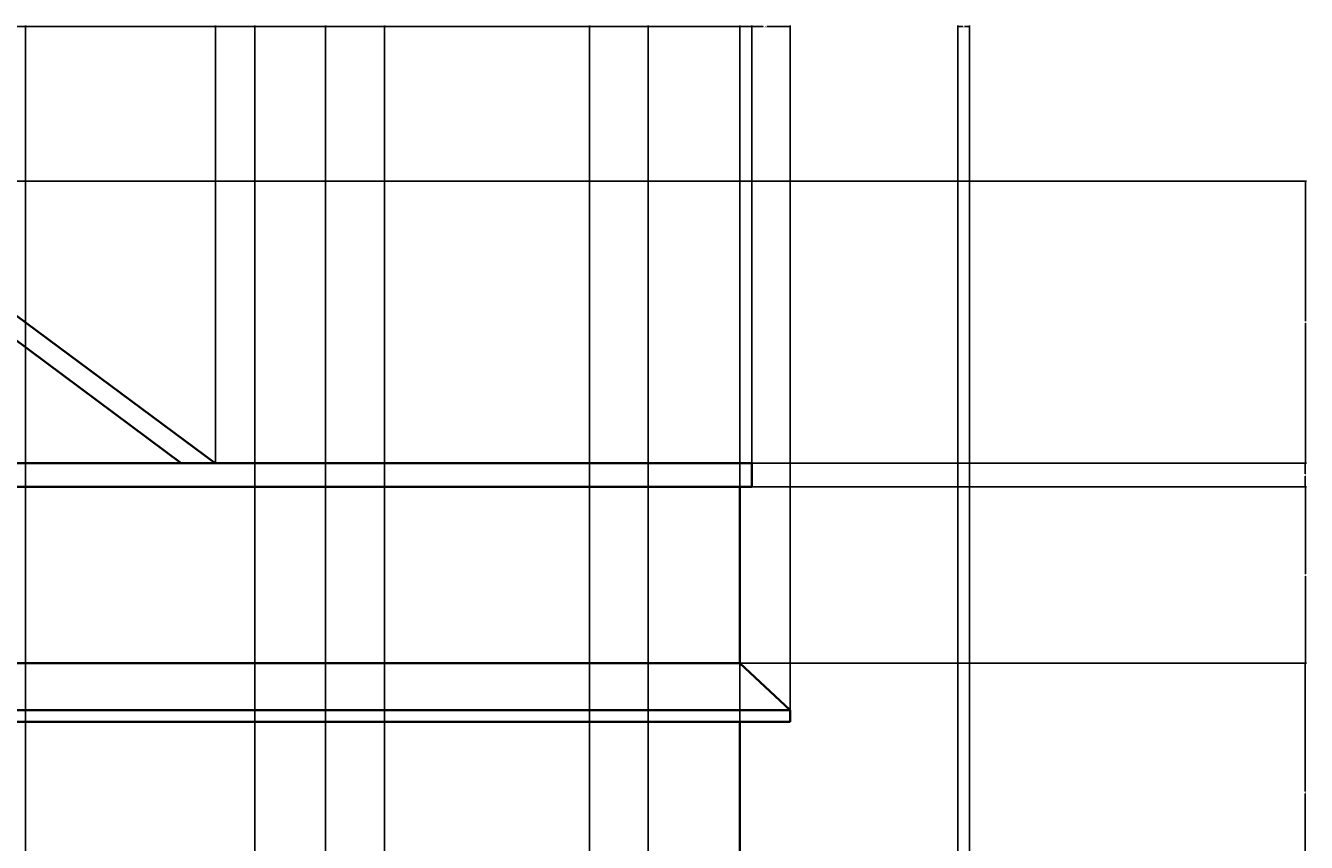
# Model space of a CAD drawing. Units: inches. Extents: x 1817 to 2378, y 1915 to 2370.
# Tile 8 of 8: x 2160 to 2377, y 2231 to 2370. Entities that reach past the tile are written whole.
import ezdxf

# ---------------------------------------------------------------- set-up
doc = ezdxf.new("R2010")
doc.units = ezdxf.units.IN
doc.layers.add('A-ANNO-DIMS', color=2, linetype='Continuous', lineweight=18)
doc.layers.add('A-ELEV', color=7, linetype='Continuous', lineweight=35)
doc.styles.get("Standard").update_dxf_attribs({"font": 'arial.ttf'})
doc.dimstyles.get("Standard").update_dxf_attribs({"dimtxt": 0.18, "dimasz": 0.18, "dimexe": 0.18, "dimexo": 0.0625, "dimgap": 0.09, "dimtad": 0, "dimtih": 1, "dimtoh": 1, "dimdec": 4, "dimzin": 0, "dimdsep": 46, "dimtxsty": 'Standard', "dimcen": 0.09, "dimadec": 0, "dimazin": 0, "dimtfac": 1, "dimtdec": 4, "dimtofl": 0, "dimtmove": 0, "dimatfit": 3, "dimfxl": 1, "dimtolj": 1, "dimtzin": 0, "dimarcsym": 0})

# ---------------------------------------------------------------- blocks, each defined once
blk = doc.blocks.new('*D36')
at = {"layer": 'A-ANNO-DIMS', "color": 0, "lineweight": -2, "transparency": 16777216}
for p, q in [((2159.62, 2217.96), (2159.62, 2369.94)), ((2159.8, 2369.76), (2178.71, 2369.76)), ((2198.41, 2369.76), (2179.5, 2369.76)), ((2198.59, 2156.58), (2198.59, 2369.94))]:
    blk.add_line(p, q, dxfattribs=at)
at = {"layer": 'A-ANNO-DIMS', "color": 0, "transparency": 16777216}
for points in [[(2159.8, 2369.79), (2159.8, 2369.73), (2159.62, 2369.76)], [(2198.41, 2369.79), (2198.41, 2369.73), (2198.59, 2369.76)]]:
    blk.add_solid(points, dxfattribs=at)
at = {"layer": 'Defpoints', "color": 0, "transparency": 16777216}
for p in [(2198.59, 2369.76), (2159.62, 2217.9), (2198.59, 2156.51)]:
    blk.add_point(p, dxfattribs=at)
at = {"layer": 'A-ANNO-DIMS', "color": 0, "transparency": 16777216, "insert": (2179.1, 2369.76), "char_height": 0.18, "attachment_point": 5}
blk.add_mtext('\\A1;38.97', dxfattribs=at)
blk = doc.blocks.new('*D37')
at = {"layer": 'A-ANNO-DIMS', "color": 0, "lineweight": -2, "transparency": 16777216}
for p, q in [((2198.59, 2156.58), (2198.59, 2369.94)), ((2198.77, 2369.76), (2204.15, 2369.76)), ((2210.44, 2369.76), (2205.06, 2369.76)), ((2210.62, 2217.57), (2210.62, 2369.94))]:
    blk.add_line(p, q, dxfattribs=at)
at = {"layer": 'A-ANNO-DIMS', "color": 0, "transparency": 16777216}
for points in [[(2198.77, 2369.79), (2198.77, 2369.73), (2198.59, 2369.76)], [(2210.44, 2369.79), (2210.44, 2369.73), (2210.62, 2369.76)]]:
    blk.add_solid(points, dxfattribs=at)
at = {"layer": 'Defpoints', "color": 0, "transparency": 16777216}
for p in [(2210.62, 2369.76), (2210.62, 2217.51), (2198.59, 2156.51)]:
    blk.add_point(p, dxfattribs=at)
at = {"layer": 'A-ANNO-DIMS', "color": 0, "transparency": 16777216, "insert": (2204.6, 2369.76), "char_height": 0.18, "attachment_point": 5}
blk.add_mtext('\\A1;12.027', dxfattribs=at)
blk = doc.blocks.new('*D38')
at = {"layer": 'A-ANNO-DIMS', "color": 0, "lineweight": -2, "transparency": 16777216}
for p, q in [((2210.62, 2217.57), (2210.62, 2369.94)), ((2210.8, 2369.76), (2215.41, 2369.76)), ((2220.44, 2369.76), (2215.83, 2369.76)), ((2220.62, 2136.11), (2220.62, 2369.94))]:
    blk.add_line(p, q, dxfattribs=at)
at = {"layer": 'A-ANNO-DIMS', "color": 0, "transparency": 16777216}
for points in [[(2210.8, 2369.79), (2210.8, 2369.73), (2210.62, 2369.76)], [(2220.44, 2369.79), (2220.44, 2369.73), (2220.62, 2369.76)]]:
    blk.add_solid(points, dxfattribs=at)
at = {"layer": 'Defpoints', "color": 0, "transparency": 16777216}
for p in [(2220.62, 2369.76), (2210.62, 2217.51), (2220.62, 2136.04)]:
    blk.add_point(p, dxfattribs=at)
at = {"layer": 'A-ANNO-DIMS', "color": 0, "transparency": 16777216, "insert": (2215.62, 2369.76), "char_height": 0.18, "attachment_point": 5}
blk.add_mtext('\\A1;10', dxfattribs=at)
blk = doc.blocks.new('*D39')
at = {"layer": 'A-ANNO-DIMS', "color": 0, "lineweight": -2, "transparency": 16777216}
for p, q in [((2220.62, 2136.11), (2220.62, 2369.94)), ((2220.8, 2369.76), (2237.66, 2369.76)), ((2255.31, 2369.76), (2238.45, 2369.76)), ((2255.49, 2136.11), (2255.49, 2369.94))]:
    blk.add_line(p, q, dxfattribs=at)
at = {"layer": 'A-ANNO-DIMS', "color": 0, "transparency": 16777216}
for points in [[(2220.8, 2369.79), (2220.8, 2369.73), (2220.62, 2369.76)], [(2255.31, 2369.79), (2255.31, 2369.73), (2255.49, 2369.76)]]:
    blk.add_solid(points, dxfattribs=at)
at = {"layer": 'Defpoints', "color": 0, "transparency": 16777216}
for p in [(2255.49, 2369.76), (2220.62, 2136.04), (2255.49, 2136.04)]:
    blk.add_point(p, dxfattribs=at)
at = {"layer": 'A-ANNO-DIMS', "color": 0, "transparency": 16777216, "insert": (2238.05, 2369.76), "char_height": 0.18, "attachment_point": 5}
blk.add_mtext('\\A1;34.87', dxfattribs=at)
blk = doc.blocks.new('*D40')
at = {"layer": 'A-ANNO-DIMS', "color": 0, "lineweight": -2, "transparency": 16777216}
for p, q in [((2255.49, 2136.11), (2255.49, 2369.94)), ((2255.67, 2369.76), (2260.28, 2369.76)), ((2265.31, 2369.76), (2260.7, 2369.76)), ((2265.49, 2217.57), (2265.49, 2369.94))]:
    blk.add_line(p, q, dxfattribs=at)
at = {"layer": 'A-ANNO-DIMS', "color": 0, "transparency": 16777216}
for points in [[(2255.67, 2369.79), (2255.67, 2369.73), (2255.49, 2369.76)], [(2265.31, 2369.79), (2265.31, 2369.73), (2265.49, 2369.76)]]:
    blk.add_solid(points, dxfattribs=at)
at = {"layer": 'Defpoints', "color": 0, "transparency": 16777216}
for p in [(2265.49, 2369.76), (2265.49, 2217.51), (2255.49, 2136.04)]:
    blk.add_point(p, dxfattribs=at)
at = {"layer": 'A-ANNO-DIMS', "color": 0, "transparency": 16777216, "insert": (2260.49, 2369.76), "char_height": 0.18, "attachment_point": 5}
blk.add_mtext('\\A1;10', dxfattribs=at)
blk = doc.blocks.new('*D41')
at = {"layer": 'A-ANNO-DIMS', "color": 0, "lineweight": -2, "transparency": 16777216}
for p, q in [((2318.11, 2103.63), (2318.11, 2369.94)), ((2318.29, 2369.76), (2318.96, 2369.76)), ((2319.93, 2369.76), (2319.26, 2369.76)), ((2320.11, 2156.58), (2320.11, 2369.94))]:
    blk.add_line(p, q, dxfattribs=at)
at = {"layer": 'A-ANNO-DIMS', "color": 0, "transparency": 16777216}
for points in [[(2318.29, 2369.79), (2318.29, 2369.73), (2318.11, 2369.76)], [(2319.93, 2369.79), (2319.93, 2369.73), (2320.11, 2369.76)]]:
    blk.add_solid(points, dxfattribs=at)
at = {"layer": 'Defpoints', "color": 0, "transparency": 16777216}
for p in [(2320.11, 2369.76), (2320.11, 2156.51), (2318.11, 2103.57)]:
    blk.add_point(p, dxfattribs=at)
at = {"layer": 'A-ANNO-DIMS', "color": 0, "transparency": 16777216, "insert": (2319.11, 2369.76), "char_height": 0.18, "attachment_point": 5}
blk.add_mtext('\\A1;2', dxfattribs=at)
blk = doc.blocks.new('*D47')
at = {"layer": 'A-ANNO-DIMS', "color": 0, "lineweight": -2, "transparency": 16777216}
for p, q in [((2127.08, 2343.57), (2127.08, 2369.94)), ((2127.26, 2369.76), (2159.09, 2369.76)), ((2191.7, 2369.76), (2159.87, 2369.76)), ((2191.88, 2295.57), (2191.88, 2369.94))]:
    blk.add_line(p, q, dxfattribs=at)
at = {"layer": 'A-ANNO-DIMS', "color": 0, "transparency": 16777216}
for points in [[(2127.26, 2369.79), (2127.26, 2369.73), (2127.08, 2369.76)], [(2191.7, 2369.79), (2191.7, 2369.73), (2191.88, 2369.76)]]:
    blk.add_solid(points, dxfattribs=at)
at = {"layer": 'Defpoints', "color": 0, "transparency": 16777216}
for p in [(2191.88, 2369.76), (2127.08, 2343.51), (2191.88, 2295.51)]:
    blk.add_point(p, dxfattribs=at)
at = {"layer": 'A-ANNO-DIMS', "color": 0, "transparency": 16777216, "insert": (2159.48, 2369.76), "char_height": 0.18, "attachment_point": 5}
blk.add_mtext('\\A1;64.79', dxfattribs=at)
blk = doc.blocks.new('*D48')
at = {"layer": 'A-ANNO-DIMS', "color": 0, "lineweight": -2, "transparency": 16777216}
for p, q in [((2191.88, 2295.57), (2191.88, 2369.94)), ((2192.06, 2369.76), (2236.1, 2369.76)), ((2280.9, 2369.76), (2236.86, 2369.76)), ((2281.08, 2291.57), (2281.08, 2369.94))]:
    blk.add_line(p, q, dxfattribs=at)
at = {"layer": 'A-ANNO-DIMS', "color": 0, "transparency": 16777216}
for points in [[(2192.06, 2369.79), (2192.06, 2369.73), (2191.88, 2369.76)], [(2280.9, 2369.79), (2280.9, 2369.73), (2281.08, 2369.76)]]:
    blk.add_solid(points, dxfattribs=at)
at = {"layer": 'Defpoints', "color": 0, "transparency": 16777216}
for p in [(2281.08, 2369.76), (2191.88, 2295.51), (2281.08, 2291.51)]:
    blk.add_point(p, dxfattribs=at)
at = {"layer": 'A-ANNO-DIMS', "color": 0, "transparency": 16777216, "insert": (2236.48, 2369.76), "char_height": 0.18, "attachment_point": 5}
blk.add_mtext('\\A1;89.21', dxfattribs=at)
blk = doc.blocks.new('*D49')
at = {"layer": 'A-ANNO-DIMS', "color": 0, "lineweight": -2, "transparency": 16777216}
for p, q in [((2281.08, 2291.57), (2281.08, 2369.94)), ((2281.26, 2369.76), (2281.94, 2369.76)), ((2282.9, 2369.76), (2282.23, 2369.76)), ((2283.08, 2295.57), (2283.08, 2369.94))]:
    blk.add_line(p, q, dxfattribs=at)
at = {"layer": 'A-ANNO-DIMS', "color": 0, "transparency": 16777216}
for points in [[(2281.26, 2369.79), (2281.26, 2369.73), (2281.08, 2369.76)], [(2282.9, 2369.79), (2282.9, 2369.73), (2283.08, 2369.76)]]:
    blk.add_solid(points, dxfattribs=at)
at = {"layer": 'Defpoints', "color": 0, "transparency": 16777216}
for p in [(2283.08, 2369.76), (2283.08, 2295.51), (2281.08, 2291.51)]:
    blk.add_point(p, dxfattribs=at)
at = {"layer": 'A-ANNO-DIMS', "color": 0, "transparency": 16777216, "insert": (2282.08, 2369.76), "char_height": 0.18, "attachment_point": 5}
blk.add_mtext('\\A1;2', dxfattribs=at)
blk = doc.blocks.new('*D50')
at = {"layer": 'A-ANNO-DIMS', "color": 0, "lineweight": -2, "transparency": 16777216}
for p, q in [((2281.08, 2261.57), (2281.08, 2369.94)), ((2281.26, 2369.76), (2285.02, 2369.76)), ((2289.43, 2369.76), (2285.67, 2369.76)), ((2289.61, 2253.57), (2289.61, 2369.94))]:
    blk.add_line(p, q, dxfattribs=at)
at = {"layer": 'A-ANNO-DIMS', "color": 0, "transparency": 16777216}
for points in [[(2281.26, 2369.79), (2281.26, 2369.73), (2281.08, 2369.76)], [(2289.43, 2369.79), (2289.43, 2369.73), (2289.61, 2369.76)]]:
    blk.add_solid(points, dxfattribs=at)
at = {"layer": 'Defpoints', "color": 0, "transparency": 16777216}
for p in [(2289.61, 2369.76), (2281.08, 2261.51), (2289.61, 2253.51)]:
    blk.add_point(p, dxfattribs=at)
at = {"layer": 'A-ANNO-DIMS', "color": 0, "transparency": 16777216, "insert": (2285.35, 2369.76), "char_height": 0.18, "attachment_point": 5}
blk.add_mtext('\\A1;8.52', dxfattribs=at)
blk = doc.blocks.new('*D51')
at = {"layer": 'A-ANNO-DIMS', "color": 0, "lineweight": -2, "transparency": 16777216}
for p, q in [((2281.02, 2261.51), (1817.4, 2261.51)), ((1817.58, 2261.33), (1817.58, 2257.69)), ((1817.58, 2253.69), (1817.58, 2257.33)), ((2289.54, 2253.51), (1817.4, 2253.51))]:
    blk.add_line(p, q, dxfattribs=at)
at = {"layer": 'A-ANNO-DIMS', "color": 0, "transparency": 16777216}
for points in [[(1817.55, 2261.33), (1817.61, 2261.33), (1817.58, 2261.51)], [(1817.55, 2253.69), (1817.61, 2253.69), (1817.58, 2253.51)]]:
    blk.add_solid(points, dxfattribs=at)
at = {"layer": 'Defpoints', "color": 0, "transparency": 16777216}
for p in [(1817.58, 2261.51), (2281.08, 2261.51), (2289.61, 2253.51)]:
    blk.add_point(p, dxfattribs=at)
at = {"layer": 'A-ANNO-DIMS', "color": 0, "transparency": 16777216, "insert": (1817.58, 2257.51), "char_height": 0.18, "attachment_point": 5}
blk.add_mtext('\\A1;8', dxfattribs=at)
blk = doc.blocks.new('*D76')
at = {"layer": 'A-ANNO-DIMS', "color": 0, "lineweight": -2, "transparency": 16777216}
for p, q in [((2281.147352, 2261.508728), (2377.398057, 2261.508728)), ((2377.218057, 2261.328728), (2377.218057, 2239.688728)), ((2377.218057, 2217.688728), (2377.218057, 2239.328728)), ((2265.550872, 2217.508728), (2377.398057, 2217.508728))]:
    blk.add_line(p, q, dxfattribs=at)
at = {"layer": 'A-ANNO-DIMS', "color": 0, "transparency": 16777216}
for points in [[(2377.188057, 2261.328728), (2377.248057, 2261.328728), (2377.218057, 2261.508728)], [(2377.188057, 2217.688728), (2377.248057, 2217.688728), (2377.218057, 2217.508728)]]:
    blk.add_solid(points, dxfattribs=at)
at = {"layer": 'Defpoints', "color": 0, "transparency": 16777216}
for p in [(2281.084852, 2261.508728), (2377.218057, 2261.508728), (2265.488372, 2217.508728)]:
    blk.add_point(p, dxfattribs=at)
at = {"layer": 'A-ANNO-DIMS', "color": 0, "transparency": 16777216, "insert": (2377.218057, 2239.508728), "char_height": 0.18, "attachment_point": 5}
blk.add_mtext('\\A1;44', dxfattribs=at)
blk = doc.blocks.new('*D77')
at = {"layer": 'A-ANNO-DIMS', "color": 0, "lineweight": -2, "transparency": 16777216}
for p, q in [((2283.15, 2291.51), (2377.4, 2291.51)), ((2377.22, 2291.33), (2377.22, 2276.69)), ((2377.22, 2261.69), (2377.22, 2276.33)), ((2281.15, 2261.51), (2377.4, 2261.51))]:
    blk.add_line(p, q, dxfattribs=at)
at = {"layer": 'A-ANNO-DIMS', "color": 0, "transparency": 16777216}
for points in [[(2377.19, 2291.33), (2377.25, 2291.33), (2377.22, 2291.51)], [(2377.19, 2261.69), (2377.25, 2261.69), (2377.22, 2261.51)]]:
    blk.add_solid(points, dxfattribs=at)
at = {"layer": 'Defpoints', "color": 0, "transparency": 16777216}
for p in [(2283.08, 2291.51), (2377.22, 2291.51), (2281.08, 2261.51)]:
    blk.add_point(p, dxfattribs=at)
at = {"layer": 'A-ANNO-DIMS', "color": 0, "transparency": 16777216, "insert": (2377.22, 2276.51), "char_height": 0.18, "attachment_point": 5}
blk.add_mtext('\\A1;30', dxfattribs=at)
blk = doc.blocks.new('*D78')
at = {"layer": 'A-ANNO-DIMS', "color": 0, "lineweight": -2, "transparency": 16777216}
for p, q in [((2283.147352, 2295.508728), (2377.398057, 2295.508728)), ((2377.218057, 2295.328728), (2377.218057, 2293.688728)), ((2377.218057, 2291.688728), (2377.218057, 2293.328728)), ((2283.147352, 2291.508728), (2377.398057, 2291.508728))]:
    blk.add_line(p, q, dxfattribs=at)
at = {"layer": 'A-ANNO-DIMS', "color": 0, "transparency": 16777216}
for points in [[(2377.188057, 2295.328728), (2377.248057, 2295.328728), (2377.218057, 2295.508728)], [(2377.188057, 2291.688728), (2377.248057, 2291.688728), (2377.218057, 2291.508728)]]:
    blk.add_solid(points, dxfattribs=at)
at = {"layer": 'Defpoints', "color": 0, "transparency": 16777216}
for p in [(2283.084852, 2295.508728), (2377.218057, 2295.508728), (2283.084852, 2291.508728)]:
    blk.add_point(p, dxfattribs=at)
at = {"layer": 'A-ANNO-DIMS', "color": 0, "transparency": 16777216, "insert": (2377.218057, 2293.508728), "char_height": 0.18, "attachment_point": 5}
blk.add_mtext('\\A1;4', dxfattribs=at)
blk = doc.blocks.new('*D79')
at = {"layer": 'A-ANNO-DIMS', "color": 0, "lineweight": -2, "transparency": 16777216}
for p, q in [((2127.15, 2343.51), (2377.4, 2343.51)), ((2377.22, 2343.33), (2377.22, 2319.69)), ((2377.22, 2295.69), (2377.22, 2319.33)), ((2283.15, 2295.51), (2377.4, 2295.51))]:
    blk.add_line(p, q, dxfattribs=at)
at = {"layer": 'A-ANNO-DIMS', "color": 0, "transparency": 16777216}
for points in [[(2377.19, 2343.33), (2377.25, 2343.33), (2377.22, 2343.51)], [(2377.19, 2295.69), (2377.25, 2295.69), (2377.22, 2295.51)]]:
    blk.add_solid(points, dxfattribs=at)
at = {"layer": 'Defpoints', "color": 0, "transparency": 16777216}
for p in [(2127.08, 2343.51), (2377.22, 2343.51), (2283.08, 2295.51)]:
    blk.add_point(p, dxfattribs=at)
at = {"layer": 'A-ANNO-DIMS', "color": 0, "transparency": 16777216, "insert": (2377.22, 2319.51), "char_height": 0.18, "attachment_point": 5}
blk.add_mtext('\\A1;48', dxfattribs=at)
blk = doc.blocks.new('*D119')
at = {"layer": 'A-ANNO-DIMS', "color": 0, "lineweight": -2, "transparency": 16777216}
for p, q in [((1903.08, 1989.57), (1903.08, 2369.94)), ((1903.26, 2369.76), (2091.62, 2369.76)), ((2280.9, 2369.76), (2092.55, 2369.76)), ((2281.08, 1989.57), (2281.08, 2369.94))]:
    blk.add_line(p, q, dxfattribs=at)
at = {"layer": 'A-ANNO-DIMS', "color": 0, "transparency": 16777216}
for points in [[(1903.26, 2369.79), (1903.26, 2369.73), (1903.08, 2369.76)], [(2280.9, 2369.79), (2280.9, 2369.73), (2281.08, 2369.76)]]:
    blk.add_solid(points, dxfattribs=at)
at = {"layer": 'Defpoints', "color": 0, "transparency": 16777216}
for p in [(2281.08, 2369.76), (1903.08, 1989.51), (2281.08, 1989.51)]:
    blk.add_point(p, dxfattribs=at)
at = {"layer": 'A-ANNO-DIMS', "color": 0, "transparency": 16777216, "insert": (2092.08, 2369.76), "char_height": 0.18, "attachment_point": 5}
blk.add_mtext('\\A1;378.00', dxfattribs=at)

msp = doc.modelspace()

# ---------------------------------------------------------------- linework, layer by layer
at = {"layer": 'A-ELEV'}
for p, q in [((2191.8757, 2295.5087), (2127.0849, 2343.5087)), ((2186.0507, 2295.5087), (2127.0849, 2339.5087)), ((2007.0849, 2295.5087), (2283.0849, 2295.5087)), ((2283.0849, 2295.5087), (2283.0849, 2291.5087)), ((2007.0849, 2291.5087), (2283.0849, 2291.5087)), ((2281.0849, 2291.5087), (2281.0849, 2261.5087)), ((2281.0849, 2261.5087), (1903.0849, 2261.5087)), ((2281.0849, 2261.5087), (2289.6055, 2253.5087)), ((2289.6055, 2253.5087), (1894.506, 2253.5087)), ((2289.6055, 2253.5087), (2289.6055, 2251.5087)), ((2289.6055, 2251.5087), (1894.506, 2251.5087)), ((2281.0849, 2251.5087), (2281.0849, 1965.5087))]:
    msp.add_line(p, q, dxfattribs=at)

# ---------------------------------------------------------------- dimensions: what is measured, and where the dimension line sits
at = {"layer": 'A-ANNO-DIMS'}
for base, p1, p2, override, picture, middle in [((2281.0849, 2369.7587), (1903.0849, 1989.5087), (2281.0849, 1989.5087), {"dimdec": 2, "dimlfac": 1, "dimrnd": 0, "dimzin": 0, "dimdsep": 46, "dimlunit": 2}, '*D119', (2092.0849, 2369.7587)), ((2191.8757, 2369.7587), (2127.0849, 2343.5087), (2191.8757, 2295.5087), {"dimdec": 2, "dimlfac": 1, "dimrnd": 0, "dimzin": 0, "dimdsep": 46, "dimlunit": 2}, '*D47', (2159.4803, 2369.7587)), ((2198.5896, 2369.7587), (2159.6179, 2217.8955), (2198.5896, 2156.5133), {"dimdec": 2, "dimlfac": 1, "dimrnd": 0, "dimzin": 0, "dimdsep": 46, "dimlunit": 2}, '*D36', (2179.1037, 2369.7587)), ((2281.0849, 2369.7587), (2191.8757, 2295.5087), (2281.0849, 2291.5087), {"dimdec": 2, "dimlfac": 1, "dimrnd": 0, "dimzin": 0, "dimdsep": 46, "dimlunit": 2}, '*D48', (2236.4803, 2369.7587)), ((2210.6163, 2369.7587), (2198.5896, 2156.5133), (2210.6163, 2217.5087), {"dimdec": 3, "dimlfac": 1, "dimrnd": 0, "dimzin": 0, "dimdsep": 46, "dimlunit": 2}, '*D37', (2204.6029, 2369.7587)), ((2220.6163, 2369.7587), (2210.6163, 2217.5087), (2220.6163, 2136.0427), {"dimdec": 0, "dimlfac": 1, "dimrnd": 0, "dimzin": 0, "dimdsep": 46, "dimlunit": 2}, '*D38', (2215.6163, 2369.7587)), ((2255.4884, 2369.7587), (2220.6163, 2136.0427), (2255.4884, 2136.0427), {"dimdec": 2, "dimlfac": 1, "dimrnd": 0, "dimzin": 0, "dimdsep": 46, "dimlunit": 2}, '*D39', (2238.0523, 2369.7587)), ((2265.4884, 2369.7587), (2255.4884, 2136.0427), (2265.4884, 2217.5087), {"dimdec": 0, "dimlfac": 1, "dimrnd": 0, "dimzin": 0, "dimdsep": 46, "dimlunit": 2}, '*D40', (2260.4884, 2369.7587)), ((2283.0849, 2369.7587), (2281.0849, 2291.5087), (2283.0849, 2295.5087), {"dimdec": 0, "dimlfac": 1, "dimrnd": 0, "dimzin": 0, "dimdsep": 46, "dimlunit": 2}, '*D49', (2282.0849, 2369.7587)), ((2289.6055, 2369.7587), (2281.0849, 2261.5087), (2289.6055, 2253.5087), {"dimdec": 2, "dimlfac": 1, "dimrnd": 0, "dimzin": 0, "dimdsep": 46, "dimlunit": 2}, '*D50', (2285.3452, 2369.7587)), ((2320.1054, 2369.7587), (2318.1054, 2103.5721), (2320.1054, 2156.5133), {"dimdec": 0, "dimlfac": 1, "dimrnd": 0, "dimzin": 0, "dimdsep": 46, "dimlunit": 2}, '*D41', (2319.1054, 2369.7587))]:
    dim = msp.add_linear_dim(base=base, p1=p1, p2=p2, dimstyle='Standard', override=override, dxfattribs=at)
    dim.commit()
    dim.dimension.update_dxf_attribs({"geometry": picture, "text_midpoint": middle})
for base, p1, p2, picture, middle in [((2377.2181, 2343.5087), (2283.0849, 2295.5087), (2127.0849, 2343.5087), '*D79', (2377.2181, 2319.5087)), ((2377.2181, 2295.5087), (2283.0849, 2291.5087), (2283.0849, 2295.5087), '*D78', (2377.2181, 2293.5087)), ((2377.2181, 2291.5087), (2281.0849, 2261.5087), (2283.0849, 2291.5087), '*D77', (2377.2181, 2276.5087)), ((1817.584, 2261.5087), (2289.6055, 2253.5087), (2281.0849, 2261.5087), '*D51', (1817.584, 2257.5087)), ((2377.2181, 2261.5087), (2265.4884, 2217.5087), (2281.0849, 2261.5087), '*D76', (2377.2181, 2239.5087))]:
    dim = msp.add_linear_dim(base=base, p1=p1, p2=p2, angle=90, dimstyle='Standard', override={"dimdec": 0, "dimlfac": 1, "dimrnd": 0, "dimzin": 0, "dimdsep": 46, "dimlunit": 2}, dxfattribs=at)
    dim.commit()
    dim.dimension.update_dxf_attribs({"geometry": picture, "text_midpoint": middle})

doc.saveas('drawing.dxf')
